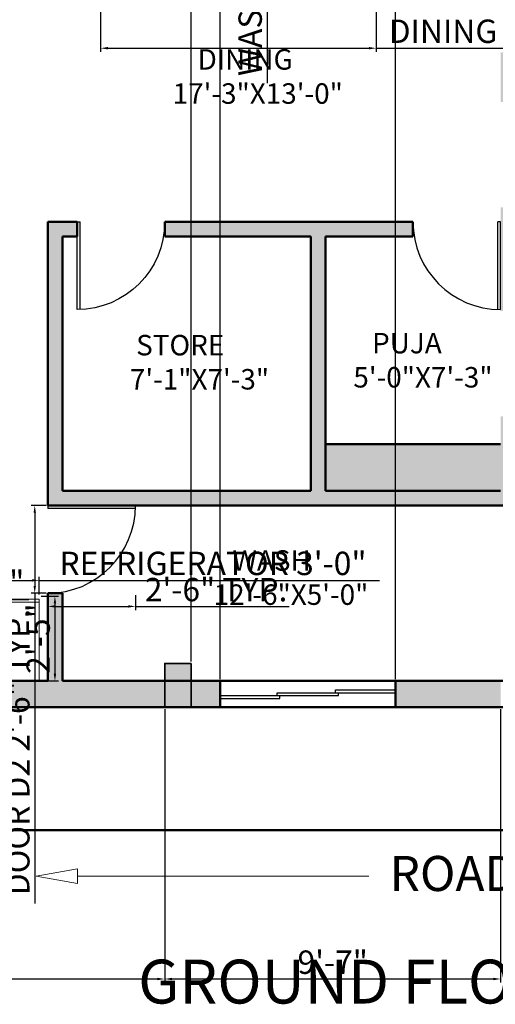
# Model space of a CAD drawing. Units: inches. Extents: x 1770 to 3141, y 984 to 1614.
# Tile 2 of 12: x 1952 to 2115, y 984 to 1320. Entities that reach past the tile are written whole.
import ezdxf

# ---------------------------------------------------------------- set-up
doc = ezdxf.new("R2010")
doc.units = ezdxf.units.IN
for name, color, linetype, lineweight in [('A-ANNO-DIMS', 2, 'Continuous', 18), ('A-ANNO-SYMB', 7, 'Continuous', 18), ('A-ANNO-TEXT', 7, 'Continuous', 18), ('A-AREA-IDEN', 3, 'Continuous', 18), ('A-COLS', 1, 'Continuous', 35), ('A-DOOR', 4, 'Continuous', 25), ('A-FLOR-FIXT', 8, 'Continuous', 18), ('A-GLAZ', 5, 'Continuous', 25), ('A-WALL', 7, 'Continuous', 50), ('A-WALL-PATT', 8, 'Continuous', 13)]:
    doc.layers.add(name, color=color, linetype=linetype, lineweight=lineweight)
doc.styles.get("Standard").update_dxf_attribs({"font": 'arial.ttf'})
doc.dimstyles.new('ISO-25', dxfattribs={"dimtxt": 8, "dimasz": 2.5, "dimexe": 1.25, "dimexo": 0.625, "dimtad": 1, "dimdec": 1, "dimlunit": 3, "dimtxsty": 'Standard', "dimcen": 2.5, "dimclrt": 1, "dimadec": 0, "dimazin": 0, "dimtfac": 1, "dimtdec": 1, "dimtmove": 0, "dimatfit": 3, "dimfxl": 1, "dimarcsym": 0})

# ---------------------------------------------------------------- blocks, each defined once
blk = doc.blocks.new("D2 2'6")
for p, q in [((0, 30), (0, 0)), ((1, 30), (1, 0)), ((0, 0), (1, 0))]:
    blk.add_line(p, q)
blk.add_arc((0, 0), 30, 0, 90)
blk = doc.blocks.new('Refrigerator-2 door - 36 in top')
for p, q in [((0, -26.999999), (36, -26.999999)), ((11, -27.999999), (11, -28.999999)), ((11, -28.999999), (13, -28.999999)), ((12, -26.999999), (12, -28.999999)), ((13, -28.999999), (13, -27.999999))]:
    blk.add_line(p, q)
blk.add_lwpolyline([(0, -27.999999), (0, 0), (36, 0), (36, -27.999999)], close=True)
blk = doc.blocks.new('COLUMN-9x15')
at = {"transparency": 33554687}
h = blk.add_hatch(color=256, dxfattribs=at)
h.dxf.hatch_style = 1
h.paths.add_polyline_path([(9, 15), (0, 15), (0, 0), (9, 0)])
blk.add_lwpolyline([(9, 15), (0, 15), (0, 0), (9, 0)], close=True)
blk = doc.blocks.new('*D70')
at = {"layer": 'A-ANNO-DIMS', "color": 0, "lineweight": -2, "transparency": 16777216}
for p, q in [((1961.11, 1154.18), (1955.98, 1154.18)), ((1957.23, 1151.68), (1957.23, 1126.68)), ((1961.11, 1124.18), (1955.98, 1124.18)), ((1957.23, 1124.18), (1957.23, 1018.04))]:
    blk.add_line(p, q, dxfattribs=at)
at = {"layer": 'A-ANNO-DIMS', "color": 0, "transparency": 16777216}
for points in [[(1956.82, 1151.68), (1957.65, 1151.68), (1957.23, 1154.18)], [(1956.82, 1126.68), (1957.65, 1126.68), (1957.23, 1124.18)]]:
    blk.add_solid(points, dxfattribs=at)
at = {"layer": 'Defpoints', "color": 0, "transparency": 16777216}
for p in [(1961.73, 1154.18), (1957.23, 1124.18), (1961.73, 1124.18)]:
    blk.add_point(p, dxfattribs=at)
at = {"layer": 'A-ANNO-DIMS', "color": 1, "transparency": 16777216, "insert": (1952.47, 1069.86), "char_height": 8, "attachment_point": 5, "rotation": 90}
blk.add_mtext('DOOR D2 2\'-6" TYP.', dxfattribs=at)
blk = doc.blocks.new('*D71')
at = {"layer": 'A-ANNO-DIMS', "color": 0, "lineweight": -2, "transparency": 16777216}
for p, q in [((1961.73, 1123.55), (1961.73, 1118.43)), ((1991.73, 1123.55), (1991.73, 1118.43)), ((1964.23, 1119.68), (1989.23, 1119.68)), ((1991.73, 1119.68), (2044.38, 1119.68))]:
    blk.add_line(p, q, dxfattribs=at)
at = {"layer": 'A-ANNO-DIMS', "color": 0, "transparency": 16777216}
for points in [[(1964.23, 1120.1), (1964.23, 1119.26), (1961.73, 1119.68)], [(1989.23, 1120.1), (1989.23, 1119.26), (1991.73, 1119.68)]]:
    blk.add_solid(points, dxfattribs=at)
at = {"layer": 'Defpoints', "color": 0, "transparency": 16777216}
for p in [(1961.73, 1124.18), (1991.73, 1124.18), (1991.73, 1119.68)]:
    blk.add_point(p, dxfattribs=at)
at = {"layer": 'A-ANNO-DIMS', "color": 1, "transparency": 16777216, "insert": (2019.31, 1124.39), "char_height": 8, "attachment_point": 5}
blk.add_mtext('2\'-6" TYP.', dxfattribs=at)
blk = doc.blocks.new('*D82')
at = {"layer": 'A-ANNO-DIMS', "color": 0, "lineweight": -2, "transparency": 16777216}
for p, q in [((1853.23, 1117.3), (1853.23, 1123.33)), ((1855.73, 1122.08), (1886.73, 1122.08)), ((1889.23, 1117.3), (1889.23, 1123.33)), ((1889.23, 1122.08), (1955.2, 1122.08))]:
    blk.add_line(p, q, dxfattribs=at)
at = {"layer": 'A-ANNO-DIMS', "color": 0, "transparency": 16777216}
for points in [[(1855.73, 1122.5), (1855.73, 1121.66), (1853.23, 1122.08)], [(1886.73, 1122.5), (1886.73, 1121.66), (1889.23, 1122.08)]]:
    blk.add_solid(points, dxfattribs=at)
at = {"layer": 'Defpoints', "color": 0, "transparency": 16777216}
for p in [(1889.23, 1122.08), (1853.23, 1116.68), (1889.23, 1116.68)]:
    blk.add_point(p, dxfattribs=at)
at = {"layer": 'A-ANNO-DIMS', "color": 1, "transparency": 16777216, "insert": (1923.47, 1126.85), "char_height": 8, "attachment_point": 5}
blk.add_mtext('STOVE 3\'-0"', dxfattribs=at)
blk = doc.blocks.new('*D86')
at = {"layer": 'A-ANNO-DIMS', "color": 0, "lineweight": -2, "transparency": 16777216}
for p, q in [((1922.74, 1123.8), (1922.74, 1129.83)), ((1925.24, 1128.58), (1956.24, 1128.58)), ((1958.74, 1123.8), (1958.74, 1129.83)), ((1958.74, 1128.58), (2075.24, 1128.58))]:
    blk.add_line(p, q, dxfattribs=at)
at = {"layer": 'A-ANNO-DIMS', "color": 0, "transparency": 16777216}
for points in [[(1925.24, 1129), (1925.24, 1128.16), (1922.74, 1128.58)], [(1956.24, 1129), (1956.24, 1128.16), (1958.74, 1128.58)]]:
    blk.add_solid(points, dxfattribs=at)
at = {"layer": 'Defpoints', "color": 0, "transparency": 16777216}
for p in [(1958.74, 1128.58), (1922.74, 1123.18), (1958.74, 1123.18)]:
    blk.add_point(p, dxfattribs=at)
at = {"layer": 'A-ANNO-DIMS', "color": 1, "transparency": 16777216, "insert": (2018.24, 1133.35), "char_height": 8, "attachment_point": 5}
blk.add_mtext('REFRIGERATOR 3\'-0"', dxfattribs=at)
blk = doc.blocks.new('*D87')
at = {"layer": 'A-ANNO-DIMS', "color": 0, "lineweight": -2, "transparency": 16777216}
for p, q in [((1959.37, 1123.18), (1965.39, 1123.18)), ((1964.14, 1120.68), (1964.14, 1096.68)), ((1959.37, 1094.18), (1965.39, 1094.18))]:
    blk.add_line(p, q, dxfattribs=at)
at = {"layer": 'A-ANNO-DIMS', "color": 0, "transparency": 16777216}
for points in [[(1963.72, 1120.68), (1964.56, 1120.68), (1964.14, 1123.18)], [(1963.72, 1096.68), (1964.56, 1096.68), (1964.14, 1094.18)]]:
    blk.add_solid(points, dxfattribs=at)
at = {"layer": 'Defpoints', "color": 0, "transparency": 16777216}
for p in [(1958.74, 1123.18), (1958.74, 1094.18), (1964.14, 1094.18)]:
    blk.add_point(p, dxfattribs=at)
at = {"layer": 'A-ANNO-DIMS', "color": 1, "transparency": 16777216, "insert": (1959.43, 1108.68), "char_height": 8, "attachment_point": 5, "rotation": 90}
blk.add_mtext('2\'-5"', dxfattribs=at)
blk = doc.blocks.new('*D92')
at = {"layer": 'A-ANNO-DIMS', "color": 0, "lineweight": -2, "transparency": 16777216}
for p, q in [((1979.79, 1324.09), (1979.79, 1309.31)), ((2074.16, 1324.09), (2074.16, 1309.31)), ((1982.29, 1310.56), (2071.66, 1310.56)), ((2074.16, 1310.56), (2190.7, 1310.56))]:
    blk.add_line(p, q, dxfattribs=at)
at = {"layer": 'A-ANNO-DIMS', "color": 0, "transparency": 16777216}
for points in [[(1982.29, 1310.98), (1982.29, 1310.15), (1979.79, 1310.56)], [(2071.66, 1310.98), (2071.66, 1310.15), (2074.16, 1310.56)]]:
    blk.add_solid(points, dxfattribs=at)
at = {"layer": 'Defpoints', "color": 0, "transparency": 16777216}
for p in [(1979.79, 1324.72), (2074.16, 1324.72), (2074.16, 1310.56)]:
    blk.add_point(p, dxfattribs=at)
at = {"layer": 'A-ANNO-DIMS', "color": 1, "transparency": 16777216, "insert": (2133.68, 1315.32), "char_height": 8, "attachment_point": 5}
blk.add_mtext('DINING SET 7\'-10 1/2"', dxfattribs=at)
blk = doc.blocks.new('*D98')
at = {"layer": 'A-ANNO-DIMS', "color": 0, "lineweight": -2, "transparency": 16777216}
for p, q in [((2038.75, 1433.14), (2035.53, 1433.14)), ((2036.78, 1430.64), (2036.78, 1418.38)), ((2038.75, 1415.88), (2035.53, 1415.88)), ((2036.78, 1415.88), (2036.78, 1298.62))]:
    blk.add_line(p, q, dxfattribs=at)
at = {"layer": 'A-ANNO-DIMS', "color": 0, "transparency": 16777216}
for points in [[(2036.37, 1430.64), (2037.2, 1430.64), (2036.78, 1433.14)], [(2036.37, 1418.38), (2037.2, 1418.38), (2036.78, 1415.88)]]:
    blk.add_solid(points, dxfattribs=at)
at = {"layer": 'Defpoints', "color": 0, "transparency": 16777216}
for p in [(2039.37, 1433.14), (2036.78, 1415.88), (2039.37, 1415.88)]:
    blk.add_point(p, dxfattribs=at)
at = {"layer": 'A-ANNO-DIMS', "color": 1, "transparency": 16777216, "insert": (2032.02, 1356), "char_height": 8, "attachment_point": 5, "rotation": 89.9999}
blk.add_mtext('WASH BASIN 1\'-5 1/2"', dxfattribs=at)
blk = doc.blocks.new('*D110')
at = {"layer": 'A-ANNO-DIMS', "color": 0, "lineweight": -2, "transparency": 16777216}
for p, q in [((1812.73, 1084.55), (1812.73, 991.02)), ((2001.73, 1084.55), (2001.73, 991.02)), ((1815.23, 992.27), (1999.23, 992.27))]:
    blk.add_line(p, q, dxfattribs=at)
at = {"layer": 'A-ANNO-DIMS', "color": 0, "transparency": 16777216}
for points in [[(1815.23, 992.69), (1815.23, 991.85), (1812.73, 992.27)], [(1999.23, 992.69), (1999.23, 991.85), (2001.73, 992.27)]]:
    blk.add_solid(points, dxfattribs=at)
at = {"layer": 'Defpoints', "color": 0, "transparency": 16777216}
for p in [(1812.73, 1085.18), (2001.73, 1085.18), (2001.73, 992.27)]:
    blk.add_point(p, dxfattribs=at)
at = {"layer": 'A-ANNO-DIMS', "color": 1, "transparency": 16777216, "insert": (1907.23, 996.98), "char_height": 8, "attachment_point": 5}
blk.add_mtext('15\'-9"', dxfattribs=at)
blk = doc.blocks.new('*D111')
at = {"layer": 'A-ANNO-DIMS', "color": 0, "lineweight": -2, "transparency": 16777216}
for p, q in [((2001.73, 1084.55), (2001.73, 991.02)), ((2116.73, 1084.55), (2116.73, 991.02)), ((2004.23, 992.27), (2114.23, 992.27))]:
    blk.add_line(p, q, dxfattribs=at)
at = {"layer": 'A-ANNO-DIMS', "color": 0, "transparency": 16777216}
for points in [[(2004.23, 992.69), (2004.23, 991.85), (2001.73, 992.27)], [(2114.23, 992.69), (2114.23, 991.85), (2116.73, 992.27)]]:
    blk.add_solid(points, dxfattribs=at)
at = {"layer": 'Defpoints', "color": 0, "transparency": 16777216}
for p in [(2001.73, 1085.18), (2116.73, 1085.18), (2116.73, 992.27)]:
    blk.add_point(p, dxfattribs=at)
at = {"layer": 'A-ANNO-DIMS', "color": 1, "transparency": 16777216, "insert": (2059.23, 996.98), "char_height": 8, "attachment_point": 5}
blk.add_mtext('9\'-7"', dxfattribs=at)
blk = doc.blocks.new('*D116')
at = {"layer": 'A-ANNO-DIMS', "color": 0, "lineweight": -2, "transparency": 16777216}
for p, q in [((2010.73, 1100.8), (2010.73, 1599.03)), ((2013.23, 1597.78), (2018.19, 1597.78)), ((2020.69, 1094.8), (2020.69, 1599.03)), ((2020.69, 1597.78), (2051.92, 1597.78))]:
    blk.add_line(p, q, dxfattribs=at)
at = {"layer": 'A-ANNO-DIMS', "color": 0, "transparency": 16777216}
for points in [[(2013.23, 1598.2), (2013.23, 1597.36), (2010.73, 1597.78)], [(2018.19, 1598.2), (2018.19, 1597.36), (2020.69, 1597.78)]]:
    blk.add_solid(points, dxfattribs=at)
at = {"layer": 'Defpoints', "color": 0, "transparency": 16777216}
for p in [(2020.69, 1597.78), (2010.73, 1100.18), (2020.69, 1094.18)]:
    blk.add_point(p, dxfattribs=at)
at = {"layer": 'A-ANNO-DIMS', "color": 1, "transparency": 16777216, "insert": (2037.56, 1602.49), "char_height": 8, "attachment_point": 5}
blk.add_mtext('0\'-10"', dxfattribs=at)
blk = doc.blocks.new('*D117')
at = {"layer": 'A-ANNO-DIMS', "color": 0, "lineweight": -2, "transparency": 16777216}
for p, q in [((2020.69, 1094.8), (2020.69, 1599.03)), ((2023.19, 1597.78), (2078.19, 1597.78)), ((2080.69, 1094.8), (2080.69, 1599.03))]:
    blk.add_line(p, q, dxfattribs=at)
at = {"layer": 'A-ANNO-DIMS', "color": 0, "transparency": 16777216}
for points in [[(2023.19, 1598.2), (2023.19, 1597.36), (2020.69, 1597.78)], [(2078.19, 1598.2), (2078.19, 1597.36), (2080.69, 1597.78)]]:
    blk.add_solid(points, dxfattribs=at)
at = {"layer": 'Defpoints', "color": 0, "transparency": 16777216}
for p in [(2080.69, 1597.78), (2020.69, 1094.18), (2080.69, 1094.18)]:
    blk.add_point(p, dxfattribs=at)
at = {"layer": 'A-ANNO-DIMS', "color": 1, "transparency": 16777216, "insert": (2050.69, 1602.49), "char_height": 8, "attachment_point": 5}
blk.add_mtext('5\'-0"', dxfattribs=at)

msp = doc.modelspace()

# ---------------------------------------------------------------- hatches: boundary and pattern name
at = {"layer": 'A-WALL-PATT'}
h = msp.add_hatch(color=256, dxfattribs=at)
h.dxf.hatch_style = 1
h.paths.add_polyline_path([(1821.73, 1556.18), (1844.25, 1556.18), (2086.73, 1556.18), (2086.73, 1443.18), (2091.73, 1443.18), (2091.73, 1556.18), (2239.73, 1556.18), (2239.73, 1565.18), (1812.73, 1565.18), (1812.73, 1100.18), (1821.73, 1100.18), (1821.73, 1246.18), (1913.73, 1246.18), (1913.73, 1251.18), (1821.73, 1251.18), (1821.73, 1407.18), (1944.73, 1407.18), (1944.73, 1412.18), (1821.73, 1412.18)])
h.paths.add_polyline_path([(1985.73, 1515.18), (1997.73, 1515.18), (1997.73, 1520.18), (1980.73, 1520.18), (1980.73, 1478.18), (1985.73, 1478.18)], flags=16)
h.paths.add_polyline_path([(2038.73, 1520.18), (2021.73, 1520.18), (2021.73, 1515.18), (2033.73, 1515.18), (2033.73, 1412.18), (1985.73, 1412.18), (1985.73, 1448.18), (1980.73, 1448.18), (1980.73, 1407.18), (2038.73, 1407.18), (2038.73, 1443.18), (2056.73, 1443.18), (2056.73, 1448.18), (2038.73, 1448.18)], flags=17)
h.paths.add_polyline_path([(1853.23, 1094.18), (1821.73, 1094.18), (1821.73, 1085.18), (1853.23, 1085.18)])
h.paths.add_polyline_path([(2001.73, 1094.18), (1966.73, 1094.18), (1966.73, 1124.18), (1961.73, 1124.18), (1961.73, 1094.18), (1889.23, 1094.18), (1889.23, 1085.18), (2001.73, 1085.18)])
h.paths.add_polyline_path([(2020.69, 1094.18), (2010.73, 1094.18), (2010.73, 1085.18), (2020.69, 1085.18)])
h.paths.add_polyline_path([(2116.73, 1094.18), (2080.69, 1094.18), (2080.69, 1085.18), (2116.73, 1085.18)])
h.paths.add_polyline_path([(2125.73, 1184.68), (2116.73, 1184.68), (2116.73, 1159.18), (2056.73, 1159.18), (2056.73, 1246.18), (2086.73, 1246.18), (2086.73, 1251.18), (2001.73, 1251.18), (2001.73, 1246.18), (2051.73, 1246.18), (2051.73, 1159.18), (1966.73, 1159.18), (1966.73, 1246.18), (1971.73, 1246.18), (1971.73, 1251.18), (1961.73, 1251.18), (1961.73, 1154.18), (1991.73, 1154.18), (2125.73, 1154.18)], flags=17)
h.paths.add_polyline_path([(2125.73, 1256.18), (2116.73, 1256.18), (2116.73, 1220.68), (2125.73, 1220.68)], flags=17)
h.paths.add_polyline_path([(2128.73, 1309.18), (2116.73, 1309.18), (2116.73, 1292.18), (2125.73, 1292.18), (2125.73, 1300.18), (2128.73, 1300.18)], flags=17)
h.paths.add_polyline_path([(2239.73, 1309.18), (2217.73, 1309.18), (2217.73, 1300.18), (2239.73, 1300.18)], flags=17)
h.paths.add_polyline_path([(2181.73, 1309.18), (2176.73, 1309.18), (2176.73, 1300.18), (2181.73, 1300.18)], flags=17)
h = msp.add_hatch(color=256, dxfattribs=at)
h.dxf.hatch_style = 1
h.paths.add_polyline_path([(2116.73, 1175.18), (2056.73, 1175.18), (2056.73, 1159.18), (2116.73, 1159.18)])

# ---------------------------------------------------------------- linework, layer by layer
at = {"layer": 'A-ANNO-SYMB'}
msp.add_line((1971.84, 1027.42), (2071.66, 1027.42), dxfattribs=at)
msp.add_lwpolyline([(1957.68, 1027.42), (1971.84, 1029.98), (1971.84, 1024.87)], close=True, dxfattribs=at)
at = {"layer": 'A-GLAZ'}
for p, q in [((2060.19, 1091.18), (2080.69, 1091.18)), ((2060.19, 1090.18), (2060.19, 1091.18)), ((2020.69, 1089.18), (2061.19, 1089.18)), ((2020.69, 1088.18), (2041.19, 1088.18)), ((2040.19, 1090.18), (2080.69, 1090.18)), ((2040.19, 1089.18), (2040.19, 1090.18)), ((2041.19, 1088.18), (2041.19, 1089.18)), ((2061.19, 1089.18), (2061.19, 1090.18))]:
    msp.add_line(p, q, dxfattribs=at)
at = {"layer": 'A-WALL'}
for p, q in [((1961.73, 1154.18), (1961.73, 1251.18)), ((1971.73, 1251.18), (1961.73, 1251.18)), ((1971.73, 1246.18), (1971.73, 1251.18)), ((2086.73, 1251.18), (2001.73, 1251.18)), ((2001.73, 1246.18), (2001.73, 1251.18)), ((2086.73, 1246.18), (2086.73, 1251.18)), ((1966.73, 1159.18), (1966.73, 1246.18)), ((1971.73, 1246.18), (1966.73, 1246.18)), ((2051.73, 1246.18), (2001.73, 1246.18)), ((2051.73, 1159.18), (2051.73, 1246.18)), ((2086.73, 1246.18), (2056.73, 1246.18)), ((2056.73, 1159.18), (2056.73, 1246.18)), ((2116.73, 1175.18), (2056.73, 1175.18)), ((2051.73, 1159.18), (1966.73, 1159.18)), ((2116.73, 1159.18), (2056.73, 1159.18)), ((2125.73, 1154.18), (1961.73, 1154.18)), ((1961.73, 1094.18), (1961.73, 1124.18)), ((1966.73, 1124.18), (1961.73, 1124.18)), ((1966.73, 1094.18), (1966.73, 1124.18)), ((1961.73, 1094.18), (1821.73, 1094.18)), ((2125.73, 1094.18), (1966.73, 1094.18)), ((2020.69, 1085.18), (2020.69, 1094.18)), ((2080.69, 1085.18), (2080.69, 1094.18)), ((2412.73, 1085.18), (1812.73, 1085.18)), ((2412.73, 1043.18), (1812.73, 1043.18))]:
    msp.add_line(p, q, dxfattribs=at)

# ---------------------------------------------------------------- block references
at = {"layer": 'A-COLS'}
msp.add_blockref('COLUMN-9x15', (2001.73, 1085.18), dxfattribs=at)
at = {"layer": 'A-DOOR', "xscale": -1, "rotation": 180}
msp.add_blockref("D2 2'6", (1971.73, 1251.18), dxfattribs=at)
at = {"layer": 'A-DOOR'}
for p, rotation in [((2116.73, 1251.18), 180), ((1961.73, 1154.18), 270)]:
    msp.add_blockref("D2 2'6", p, dxfattribs=dict(at, rotation=rotation))
at = {"layer": 'A-FLOR-FIXT', "xscale": -1, "rotation": 180}
msp.add_blockref('Refrigerator-2 door - 36 in top', (1922.74, 1094.18), dxfattribs=at)

# ---------------------------------------------------------------- texts
at = {"layer": 'A-ANNO-TEXT', "attachment_point": 1}
for s, width, insert, char_height in [('  ROAD', 86.9528, (2071.39, 1034.35), 12), ('GROUND FLOOR PLAN', 253.2094, (1992.64, 998.88), 15)]:
    msp.add_mtext_dynamic_manual_height_columns(s, width=width, gutter_width=12.5, heights=[0], dxfattribs=dict(at, insert=insert, char_height=char_height))
at = {"layer": 'A-AREA-IDEN', "char_height": 7, "attachment_point": 1}
for s, insert in [('    DINING \\P17\'-3"X13\'-0"', (2004.45, 1310.23)), (' STORE\\P7\'-1"X7\'-3"', (1989.8, 1212.52)), ('   PUJA\\P5\'-0"X7\'-3"', (2066.31, 1213.2)), ('   WASH \\P12\'-6"X5\'-0"', (2018.49, 1138.87))]:
    msp.add_mtext_dynamic_manual_height_columns(s, width=86.9528, gutter_width=12.5, heights=[0], dxfattribs=dict(at, insert=insert))

# ---------------------------------------------------------------- dimensions: what is measured, and where the dimension line sits
at = {"layer": 'A-ANNO-DIMS'}
for base, p1, p2, picture, middle in [((2020.69, 1597.78), (2010.73, 1100.18), (2020.69, 1094.18), '*D116', (2037.56, 1602.49)), ((2080.69, 1597.78), (2020.69, 1094.18), (2080.69, 1094.18), '*D117', (2050.69, 1602.49)), ((2001.73, 992.27), (1812.73, 1085.18), (2001.73, 1085.18), '*D110', (1907.23, 996.98)), ((2116.73, 992.27), (2001.73, 1085.18), (2116.73, 1085.18), '*D111', (2059.23, 996.98))]:
    dim = msp.add_linear_dim(base=base, p1=p1, p2=p2, dimstyle='ISO-25', override={"dimdec": 1, "dimlfac": 1, "dimrnd": 0, "dimzin": 1, "dimdsep": 46, "dimlunit": 4, "dimfrac": 2}, dxfattribs=at)
    dim.commit()
    dim.dimension.update_dxf_attribs({"geometry": picture, "text_midpoint": middle})
for base, p1, p2, angle, text, picture, middle in [((2036.78, 1415.88), (2039.37, 1433.14), (2039.37, 1415.88), 269.9999, 'WASH BASIN <>', '*D98', (2032.02, 1356)), ((1957.23, 1124.18), (1961.73, 1154.18), (1961.73, 1124.18), 270, 'DOOR D2 <> TYP.', '*D70', (1952.47, 1069.86))]:
    dim = msp.add_linear_dim(base=base, p1=p1, p2=p2, angle=angle, text=text, dimstyle='ISO-25', override={"dimdec": 1, "dimrnd": 0, "dimzin": 1, "dimlunit": 4, "dimfrac": 2}, dxfattribs=at)
    dim.commit()
    dim.dimension.update_dxf_attribs({"geometry": picture, "text_midpoint": middle})
for base, p1, p2, text, picture, middle in [((2074.16, 1310.56), (1979.79, 1324.72), (2074.16, 1324.72), 'DINING SET <>', '*D92', (2133.68, 1315.32)), ((1958.74, 1128.58), (1922.74, 1123.18), (1958.74, 1123.18), 'REFRIGERATOR <>', '*D86', (2018.24, 1133.35)), ((1889.23, 1122.08), (1853.23, 1116.68), (1889.23, 1116.68), 'STOVE <>', '*D82', (1923.47, 1126.85)), ((1991.73, 1119.68), (1961.73, 1124.18), (1991.73, 1124.18), '<> TYP.', '*D71', (2019.31, 1124.39))]:
    dim = msp.add_linear_dim(base=base, p1=p1, p2=p2, text=text, dimstyle='ISO-25', override={"dimdec": 1, "dimrnd": 0, "dimzin": 1, "dimlunit": 4, "dimfrac": 2}, dxfattribs=at)
    dim.commit()
    dim.dimension.update_dxf_attribs({"geometry": picture, "text_midpoint": middle})
dim = msp.add_linear_dim(base=(1964.14, 1094.18), p1=(1958.74, 1123.18), p2=(1958.74, 1094.18), angle=270, dimstyle='ISO-25', override={"dimdec": 1, "dimrnd": 0, "dimzin": 1, "dimlunit": 4, "dimfrac": 2}, dxfattribs=at)
dim.commit()
dim.dimension.update_dxf_attribs({"geometry": '*D87', "text_midpoint": (1959.43, 1108.68)})

doc.saveas('drawing.dxf')
